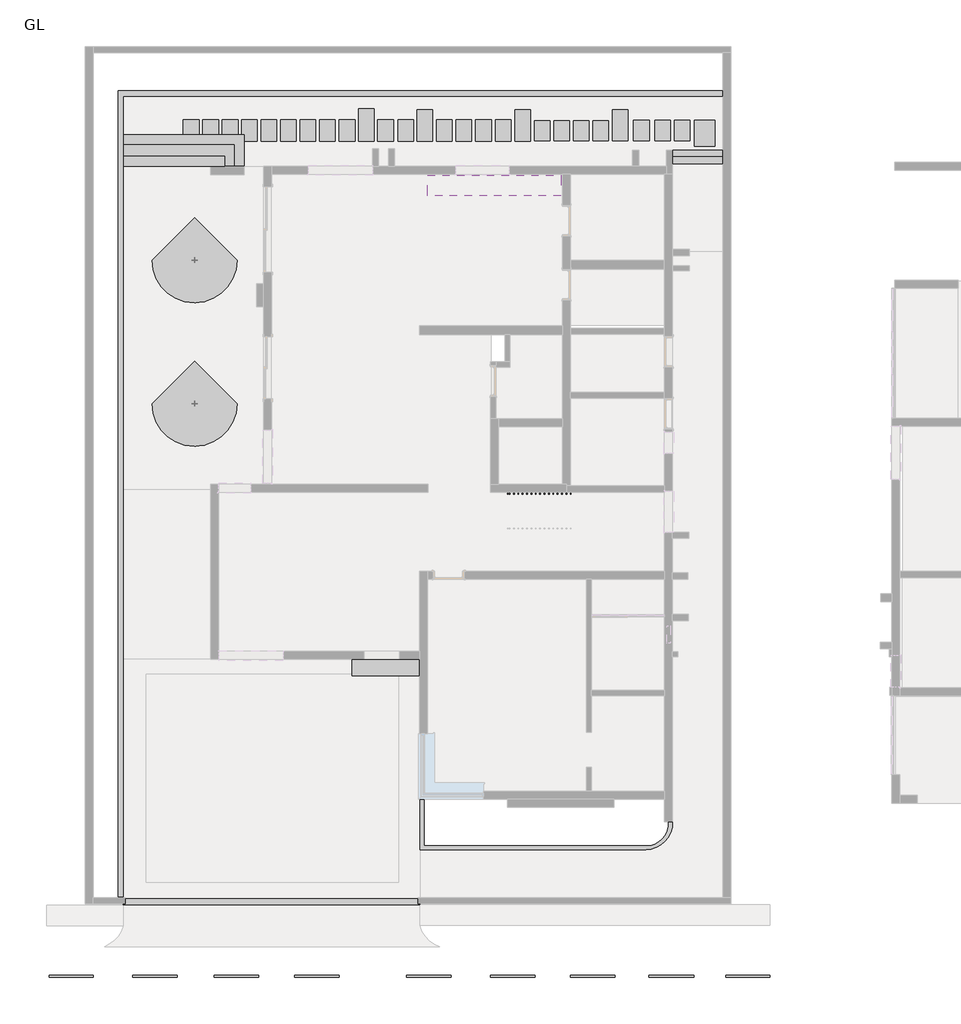
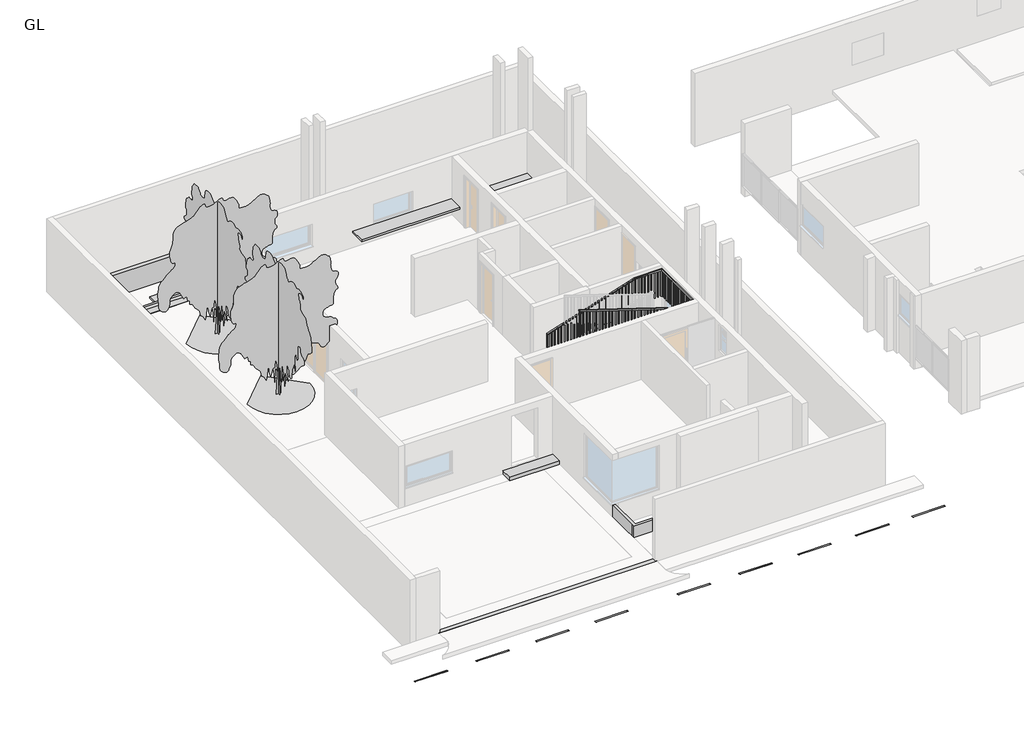
# One storey, part 6 of 6: 5 proxies, 2 geographic elements, 2 stairs, 1 railing.
"""IFC4 building model written with IfcOpenShell, lengths in millimetres."""

from ifc_helpers import new_model, si_unit, frame, origin, place, context, project, spatial, polyline, outline, extrude, faceted_brep, transform, mapped, element, save
from components import generic_models_1_generic_models_1_84634830, generic_models_2_generic_models_2_74674079, generic_models_3_generic_models_3_ad65571d, generic_models_4_generic_models_4_6f48c335, generic_models_5_generic_models_5_efa3826c, planting_rpc_tree_deciduous_golden_chain_5_5_meters_a00e3d8d, stairs_1_stairs_1_bf5218fc, stairs_2_stairs_2_b3d7acac

model = new_model("IFC4")

# Units and contexts
model_context = context("Model", 3, world=origin())
ifc_project = project(units=[si_unit("LENGTHUNIT", "METRE", prefix="MILLI")], contexts=[model_context])

# Site, building, storey
site = spatial("IfcSite", under=ifc_project)
building = spatial("IfcBuilding", under=site)
storey = spatial("IfcBuildingStorey", under=building, Name="GL", Elevation=0.0)

# Proxies
placement = place(None, origin())
generic_models_1_generic_models_1_shape = generic_models_1_generic_models_1_84634830(model_context)
element("IfcBuildingElementProxy", 1, Name="Generic Models 1 : Generic Models 1", ObjectType="Generic Models 1 : Generic Models 1", at=placement, inside=storey, context=model_context, shape_type="MappedRepresentation", body=[
    mapped(generic_models_1_generic_models_1_shape, transform((0.0, 0.0, 0.0), x_axis=(1.0, 0.0, 0.0), y_axis=(0.0, 1.0, 0.0), z_axis=(0.0, 0.0, 1.0))),
])
generic_models_2_generic_models_2_shape = generic_models_2_generic_models_2_74674079(model_context)
element("IfcBuildingElementProxy", 2, Name="Generic Models 2 : Generic Models 2", ObjectType="Generic Models 2 : Generic Models 2", at=placement, inside=storey, context=model_context, shape_type="MappedRepresentation", body=[
    mapped(generic_models_2_generic_models_2_shape, transform((0.0, 0.0, 0.0), x_axis=(1.0, 0.0, 0.0), y_axis=(0.0, 1.0, 0.0), z_axis=(0.0, 0.0, 1.0))),
])
generic_models_3_generic_models_3_shape = generic_models_3_generic_models_3_ad65571d(model_context)
element("IfcBuildingElementProxy", 3, Name="Generic Models 3 : Generic Models 3", ObjectType="Generic Models 3 : Generic Models 3", at=placement, inside=storey, context=model_context, shape_type="MappedRepresentation", body=[
    mapped(generic_models_3_generic_models_3_shape, transform((0.0, 0.0, 0.0), x_axis=(1.0, 0.0, 0.0), y_axis=(0.0, 1.0, 0.0), z_axis=(0.0, 0.0, 1.0))),
])
generic_models_4_generic_models_4_shape = generic_models_4_generic_models_4_6f48c335(model_context)
element("IfcBuildingElementProxy", 4, Name="Generic Models 4 : Generic Models 4", ObjectType="Generic Models 4 : Generic Models 4", at=placement, inside=storey, context=model_context, shape_type="MappedRepresentation", body=[
    mapped(generic_models_4_generic_models_4_shape, transform((0.0, 0.0, 0.0), x_axis=(1.0, 0.0, 0.0), y_axis=(0.0, 1.0, 0.0), z_axis=(0.0, 0.0, 1.0))),
])
generic_models_5_generic_models_5_shape = generic_models_5_generic_models_5_efa3826c(model_context)
element("IfcBuildingElementProxy", 5, Name="Generic Models 5 : Generic Models 5", ObjectType="Generic Models 5 : Generic Models 5", at=placement, inside=storey, context=model_context, shape_type="MappedRepresentation", body=[
    mapped(generic_models_5_generic_models_5_shape, transform((0.0, 0.0, 0.0), x_axis=(1.0, 0.0, 0.0), y_axis=(0.0, 1.0, 0.0), z_axis=(0.0, 0.0, 1.0))),
])

# Geographic elements
planting_rpc_tree_deciduous_golden_chain_5_5_meters_shape = planting_rpc_tree_deciduous_golden_chain_5_5_meters_a00e3d8d(model_context)
element("IfcGeographicElement", 6, ObjectType="Planting_RPC_Tree_Deciduous : Golden_Chain-5.5_Meters", at=placement, inside=storey, context=model_context, shape_type="MappedRepresentation", body=[
    mapped(planting_rpc_tree_deciduous_golden_chain_5_5_meters_shape, transform((-49097.6786333, 20390.8041063, 899.9140625), x_axis=(1.0, 0.0, 0.0), y_axis=(0.0, 1.0, 0.0), z_axis=(0.0, 0.0, 1.0))),
])
element("IfcGeographicElement", 7, ObjectType="Planting_RPC_Tree_Deciduous : Golden_Chain-5.5_Meters", at=placement, inside=storey, context=model_context, shape_type="MappedRepresentation", body=[
    mapped(planting_rpc_tree_deciduous_golden_chain_5_5_meters_shape, transform((-49097.6786333, 24492.9041063, 899.9140625), x_axis=(1.0, 0.0, 0.0), y_axis=(0.0, 1.0, 0.0), z_axis=(0.0, 0.0, 1.0))),
])

# Railing
element("IfcRailing", 8, ObjectType="1100mm", at=placement, inside=storey, context=model_context, shape_type="SolidModel", body=[
    faceted_brep([(-40149.9681829, 17835.7234223, 1799.9767904), (-40149.9681829, 17835.7234223, 1747.4487757), (-40149.9681829, 17785.7234223, 1747.4487757), (-40149.9681829, 17785.7234223, 1799.9767904), (-36733.6681829, 17835.7234223, 2899.9878906), (-36725.8169379, 17835.7234223, 2849.9878906), (-36725.8169379, 17785.7234223, 2849.9878906), (-36733.6681829, 17785.7234223, 2899.9878906), (-35651.74796, 17835.7234223, 2899.9878906), (-35651.74796, 17835.7234223, 2849.9878906), (-35701.74796, 17785.7234223, 2849.9878906), (-35701.74796, 17785.7234223, 2899.9878906), (-35651.74796, 15601.3234223, 2899.9878906), (-35651.74796, 15601.3234223, 2849.9878906), (-35701.74796, 15651.3234223, 2849.9878906), (-35701.74796, 15651.3234223, 2899.9878906), (-36423.0954556, 15601.3234223, 2899.9878906), (-36430.9467006, 15601.3234223, 2849.9878906), (-36430.9467006, 15651.3234223, 2849.9878906), (-36423.0954556, 15651.3234223, 2899.9878906), (-40149.9681829, 15601.3234223, 4100.0), (-40149.9681829, 15651.3234223, 4100.0), (-40149.9681829, 15651.3234223, 4047.4719853), (-40149.9681829, 15601.3234223, 4047.4719853)], [[[0, 1, 2, 3]], [[1, 0, 4, 5]], [[2, 1, 5, 6]], [[3, 2, 6, 7]], [[0, 3, 7, 4]], [[5, 4, 8, 9]], [[6, 5, 9, 10]], [[7, 6, 10, 11]], [[4, 7, 11, 8]], [[9, 8, 12, 13]], [[10, 9, 13, 14]], [[11, 10, 14, 15]], [[8, 11, 15, 12]], [[13, 12, 16, 17]], [[14, 13, 17, 18]], [[15, 14, 18, 19]], [[12, 15, 19, 16]], [[20, 21, 22, 23]], [[17, 16, 20, 23]], [[18, 17, 23, 22]], [[19, 18, 22, 21]], [[16, 19, 21, 20]]]),
    extrude(outline(polyline([(4031.9456028, -40101.74796), (4039.9953284, -40126.74796), (2899.9989909, -40126.74796), (2899.9989909, -40101.74796), (4031.9456028, -40101.74796)])), frame((0.0, 15613.8234223, 0.0), z_axis=(0.0, 1.0, 0.0), x_axis=(0.0, 0.0, 1.0)), (0.0, 0.0, 1.0), 25.0),
    extrude(outline(polyline([(3991.6969749, -39976.74796), (3999.7467005, -40001.74796), (2899.9989909, -40001.74796), (2899.9989909, -39976.74796), (3991.6969749, -39976.74796)])), frame((0.0, 15613.8234223, 0.0), z_axis=(0.0, 1.0, 0.0), x_axis=(0.0, 0.0, 1.0)), (0.0, 0.0, 1.0), 25.0),
    extrude(outline(polyline([(3951.448347, -39851.74796), (3959.4980726, -39876.74796), (2899.9989909, -39876.74796), (2899.9989909, -39851.74796), (3951.448347, -39851.74796)])), frame((0.0, 15613.8234223, 0.0), z_axis=(0.0, 1.0, 0.0), x_axis=(0.0, 0.0, 1.0)), (0.0, 0.0, 1.0), 25.0),
    extrude(outline(polyline([(3911.1997191, -39726.74796), (3919.2494447, -39751.74796), (2799.9979818, -39751.74796), (2799.9979818, -39726.74796), (3911.1997191, -39726.74796)])), frame((0.0, 15613.8234223, 0.0), z_axis=(0.0, 1.0, 0.0), x_axis=(0.0, 0.0, 1.0)), (0.0, 0.0, 1.0), 25.0),
    extrude(outline(polyline([(3870.9510912, -39601.74796), (3879.0008168, -39626.74796), (2799.9979818, -39626.74796), (2799.9979818, -39601.74796), (3870.9510912, -39601.74796)])), frame((0.0, 15613.8234223, 0.0), z_axis=(0.0, 1.0, 0.0), x_axis=(0.0, 0.0, 1.0)), (0.0, 0.0, 1.0), 25.0),
    extrude(outline(polyline([(3830.7024633, -39476.74796), (3838.7521889, -39501.74796), (2699.9969727, -39501.74796), (2699.9969727, -39476.74796), (3830.7024633, -39476.74796)])), frame((0.0, 15613.8234223, 0.0), z_axis=(0.0, 1.0, 0.0), x_axis=(0.0, 0.0, 1.0)), (0.0, 0.0, 1.0), 25.0),
    extrude(outline(polyline([(3790.4538354, -39351.74796), (3798.503561, -39376.74796), (2699.9969727, -39376.74796), (2699.9969727, -39351.74796), (3790.4538354, -39351.74796)])), frame((0.0, 15613.8234223, 0.0), z_axis=(0.0, 1.0, 0.0), x_axis=(0.0, 0.0, 1.0)), (0.0, 0.0, 1.0), 25.0),
    extrude(outline(polyline([(3750.2052075, -39226.74796), (3758.254933, -39251.74796), (2699.9969727, -39251.74796), (2699.9969727, -39226.74796), (3750.2052075, -39226.74796)])), frame((0.0, 15613.8234223, 0.0), z_axis=(0.0, 1.0, 0.0), x_axis=(0.0, 0.0, 1.0)), (0.0, 0.0, 1.0), 25.0),
    extrude(outline(polyline([(3710.0216346, -39101.74796), (3718.0713601, -39126.74796), (2599.9959635, -39126.74796), (2599.9959635, -39101.74796), (3710.0216346, -39101.74796)])), frame((0.0, 15613.8234223, 0.0), z_axis=(0.0, 1.0, 0.0), x_axis=(0.0, 0.0, 1.0)), (0.0, 0.0, 1.0), 25.0),
    extrude(outline(polyline([(3669.7730066, -38976.74796), (3677.8227322, -39001.74796), (2599.9959635, -39001.74796), (2599.9959635, -38976.74796), (3669.7730066, -38976.74796)])), frame((0.0, 15613.8234223, 0.0), z_axis=(0.0, 1.0, 0.0), x_axis=(0.0, 0.0, 1.0)), (0.0, 0.0, 1.0), 25.0),
    extrude(outline(polyline([(3629.5243787, -38851.74796), (3637.5741043, -38876.74796), (2499.9949544, -38876.74796), (2499.9949544, -38851.74796), (3629.5243787, -38851.74796)])), frame((0.0, 15613.8234223, 0.0), z_axis=(0.0, 1.0, 0.0), x_axis=(0.0, 0.0, 1.0)), (0.0, 0.0, 1.0), 25.0),
    extrude(outline(polyline([(3589.2757508, -38726.74796), (3597.3254764, -38751.74796), (2499.9949544, -38751.74796), (2499.9949544, -38726.74796), (3589.2757508, -38726.74796)])), frame((0.0, 15613.8234223, 0.0), z_axis=(0.0, 1.0, 0.0), x_axis=(0.0, 0.0, 1.0)), (0.0, 0.0, 1.0), 25.0),
    extrude(outline(polyline([(3549.0271229, -38601.74796), (3557.0768485, -38626.74796), (2499.9949544, -38626.74796), (2499.9949544, -38601.74796), (3549.0271229, -38601.74796)])), frame((0.0, 15613.8234223, 0.0), z_axis=(0.0, 1.0, 0.0), x_axis=(0.0, 0.0, 1.0)), (0.0, 0.0, 1.0), 25.0),
    extrude(outline(polyline([(3508.778495, -38476.74796), (3516.8282206, -38501.74796), (2399.9939453, -38501.74796), (2399.9939453, -38476.74796), (3508.778495, -38476.74796)])), frame((0.0, 15613.8234223, 0.0), z_axis=(0.0, 1.0, 0.0), x_axis=(0.0, 0.0, 1.0)), (0.0, 0.0, 1.0), 25.0),
    extrude(outline(polyline([(3468.5298671, -38351.74796), (3476.5795927, -38376.74796), (2399.9939453, -38376.74796), (2399.9939453, -38351.74796), (3468.5298671, -38351.74796)])), frame((0.0, 15613.8234223, 0.0), z_axis=(0.0, 1.0, 0.0), x_axis=(0.0, 0.0, 1.0)), (0.0, 0.0, 1.0), 25.0),
    extrude(outline(polyline([(3428.2812392, -38226.74796), (3436.3309648, -38251.74796), (2299.9929362, -38251.74796), (2299.9929362, -38226.74796), (3428.2812392, -38226.74796)])), frame((0.0, 15613.8234223, 0.0), z_axis=(0.0, 1.0, 0.0), x_axis=(0.0, 0.0, 1.0)), (0.0, 0.0, 1.0), 25.0),
    extrude(outline(polyline([(3388.0326113, -38101.74796), (3396.0823368, -38126.74796), (2299.9929362, -38126.74796), (2299.9929362, -38101.74796), (3388.0326113, -38101.74796)])), frame((0.0, 15613.8234223, 0.0), z_axis=(0.0, 1.0, 0.0), x_axis=(0.0, 0.0, 1.0)), (0.0, 0.0, 1.0), 25.0),
    extrude(outline(polyline([(3347.7839834, -37976.74796), (3355.8337089, -38001.74796), (2299.9929362, -38001.74796), (2299.9929362, -37976.74796), (3347.7839834, -37976.74796)])), frame((0.0, 15613.8234223, 0.0), z_axis=(0.0, 1.0, 0.0), x_axis=(0.0, 0.0, 1.0)), (0.0, 0.0, 1.0), 25.0),
    extrude(outline(polyline([(3307.5353554, -37851.74796), (3315.585081, -37876.74796), (2199.9919271, -37876.74796), (2199.9919271, -37851.74796), (3307.5353554, -37851.74796)])), frame((0.0, 15613.8234223, 0.0), z_axis=(0.0, 1.0, 0.0), x_axis=(0.0, 0.0, 1.0)), (0.0, 0.0, 1.0), 25.0),
    extrude(outline(polyline([(3267.2867275, -37726.74796), (3275.3364531, -37751.74796), (2199.9919271, -37751.74796), (2199.9919271, -37726.74796), (3267.2867275, -37726.74796)])), frame((0.0, 15613.8234223, 0.0), z_axis=(0.0, 1.0, 0.0), x_axis=(0.0, 0.0, 1.0)), (0.0, 0.0, 1.0), 25.0),
    extrude(outline(polyline([(3227.0380996, -37601.74796), (3235.0878252, -37626.74796), (2099.990918, -37626.74796), (2099.990918, -37601.74796), (3227.0380996, -37601.74796)])), frame((0.0, 15613.8234223, 0.0), z_axis=(0.0, 1.0, 0.0), x_axis=(0.0, 0.0, 1.0)), (0.0, 0.0, 1.0), 25.0),
    extrude(outline(polyline([(3186.7894717, -37476.74796), (3194.8391973, -37501.74796), (2099.990918, -37501.74796), (2099.990918, -37476.74796), (3186.7894717, -37476.74796)])), frame((0.0, 15613.8234223, 0.0), z_axis=(0.0, 1.0, 0.0), x_axis=(0.0, 0.0, 1.0)), (0.0, 0.0, 1.0), 25.0),
    extrude(outline(polyline([(3146.5408438, -37351.74796), (3154.5905694, -37376.74796), (2099.990918, -37376.74796), (2099.990918, -37351.74796), (3146.5408438, -37351.74796)])), frame((0.0, 15613.8234223, 0.0), z_axis=(0.0, 1.0, 0.0), x_axis=(0.0, 0.0, 1.0)), (0.0, 0.0, 1.0), 25.0),
    extrude(outline(polyline([(3106.2922159, -37226.74796), (3114.3419415, -37251.74796), (1999.9899089, -37251.74796), (1999.9899089, -37226.74796), (3106.2922159, -37226.74796)])), frame((0.0, 15613.8234223, 0.0), z_axis=(0.0, 1.0, 0.0), x_axis=(0.0, 0.0, 1.0)), (0.0, 0.0, 1.0), 25.0),
    extrude(outline(polyline([(3066.043588, -37101.74796), (3074.0933136, -37126.74796), (1999.9899089, -37126.74796), (1999.9899089, -37101.74796), (3066.043588, -37101.74796)])), frame((0.0, 15613.8234223, 0.0), z_axis=(0.0, 1.0, 0.0), x_axis=(0.0, 0.0, 1.0)), (0.0, 0.0, 1.0), 25.0),
    extrude(outline(polyline([(3025.7949601, -36976.74796), (3033.8446856, -37001.74796), (1899.9888997, -37001.74796), (1899.9888997, -36976.74796), (3025.7949601, -36976.74796)])), frame((0.0, 15613.8234223, 0.0), z_axis=(0.0, 1.0, 0.0), x_axis=(0.0, 0.0, 1.0)), (0.0, 0.0, 1.0), 25.0),
    extrude(outline(polyline([(2985.5463322, -36851.74796), (2993.5960577, -36876.74796), (1899.9888997, -36876.74796), (1899.9888997, -36851.74796), (2985.5463322, -36851.74796)])), frame((0.0, 15613.8234223, 0.0), z_axis=(0.0, 1.0, 0.0), x_axis=(0.0, 0.0, 1.0)), (0.0, 0.0, 1.0), 25.0),
    extrude(outline(polyline([(2945.2977042, -36726.74796), (2953.3474298, -36751.74796), (1899.9888997, -36751.74796), (1899.9888997, -36726.74796), (2945.2977042, -36726.74796)])), frame((0.0, 15613.8234223, 0.0), z_axis=(0.0, 1.0, 0.0), x_axis=(0.0, 0.0, 1.0)), (0.0, 0.0, 1.0), 25.0),
    extrude(outline(polyline([(2905.0490763, -36601.74796), (2913.0988019, -36626.74796), (1799.9878906, -36626.74796), (1799.9878906, -36601.74796), (2905.0490763, -36601.74796)])), frame((0.0, 15613.8234223, 0.0), z_axis=(0.0, 1.0, 0.0), x_axis=(0.0, 0.0, 1.0)), (0.0, 0.0, 1.0), 25.0),
    extrude(outline(polyline([(2864.8004484, -36476.74796), (2872.850174, -36501.74796), (1799.9878906, -36501.74796), (1799.9878906, -36476.74796), (2864.8004484, -36476.74796)])), frame((0.0, 15613.8234223, 0.0), z_axis=(0.0, 1.0, 0.0), x_axis=(0.0, 0.0, 1.0)), (0.0, 0.0, 1.0), 25.0),
    extrude(outline(polyline([(-36351.74796, 15613.8234223), (-36376.74796, 15613.8234223), (-36376.74796, 15638.8234223), (-36351.74796, 15638.8234223), (-36351.74796, 15613.8234223)])), frame((0.0, 0.0, 1799.9878906), z_axis=(0.0, 0.0, 1.0), x_axis=(1.0, 0.0, 0.0)), (0.0, 0.0, 1.0), 1050.0),
    extrude(outline(polyline([(-36226.74796, 15613.8234223), (-36251.74796, 15613.8234223), (-36251.74796, 15638.8234223), (-36226.74796, 15638.8234223), (-36226.74796, 15613.8234223)])), frame((0.0, 0.0, 1799.9878906), z_axis=(0.0, 0.0, 1.0), x_axis=(1.0, 0.0, 0.0)), (0.0, 0.0, 1.0), 1050.0),
    extrude(outline(polyline([(-36101.74796, 15613.8234223), (-36126.74796, 15613.8234223), (-36126.74796, 15638.8234223), (-36101.74796, 15638.8234223), (-36101.74796, 15613.8234223)])), frame((0.0, 0.0, 1799.9878906), z_axis=(0.0, 0.0, 1.0), x_axis=(1.0, 0.0, 0.0)), (0.0, 0.0, 1.0), 1050.0),
    extrude(outline(polyline([(-35976.74796, 15613.8234223), (-36001.74796, 15613.8234223), (-36001.74796, 15638.8234223), (-35976.74796, 15638.8234223), (-35976.74796, 15613.8234223)])), frame((0.0, 0.0, 1799.9878906), z_axis=(0.0, 0.0, 1.0), x_axis=(1.0, 0.0, 0.0)), (0.0, 0.0, 1.0), 1050.0),
    extrude(outline(polyline([(-35851.74796, 15613.8234223), (-35876.74796, 15613.8234223), (-35876.74796, 15638.8234223), (-35851.74796, 15638.8234223), (-35851.74796, 15613.8234223)])), frame((0.0, 0.0, 1799.9878906), z_axis=(0.0, 0.0, 1.0), x_axis=(1.0, 0.0, 0.0)), (0.0, 0.0, 1.0), 1050.0),
    extrude(outline(polyline([(-35726.74796, 15613.8234223), (-35751.74796, 15613.8234223), (-35751.74796, 15638.8234223), (-35726.74796, 15638.8234223), (-35726.74796, 15613.8234223)])), frame((0.0, 0.0, 1799.9878906), z_axis=(0.0, 0.0, 1.0), x_axis=(1.0, 0.0, 0.0)), (0.0, 0.0, 1.0), 1050.0),
    extrude(outline(polyline([(-35664.24796, 15760.7234223), (-35664.24796, 15735.7234223), (-35689.24796, 15735.7234223), (-35689.24796, 15760.7234223), (-35664.24796, 15760.7234223)])), frame((0.0, 0.0, 1799.9878906), z_axis=(0.0, 0.0, 1.0), x_axis=(1.0, 0.0, 0.0)), (0.0, 0.0, 1.0), 1050.0),
    extrude(outline(polyline([(-35664.24796, 15885.7234223), (-35664.24796, 15860.7234223), (-35689.24796, 15860.7234223), (-35689.24796, 15885.7234223), (-35664.24796, 15885.7234223)])), frame((0.0, 0.0, 1799.9878906), z_axis=(0.0, 0.0, 1.0), x_axis=(1.0, 0.0, 0.0)), (0.0, 0.0, 1.0), 1050.0),
    extrude(outline(polyline([(-35664.24796, 16010.7234223), (-35664.24796, 15985.7234223), (-35689.24796, 15985.7234223), (-35689.24796, 16010.7234223), (-35664.24796, 16010.7234223)])), frame((0.0, 0.0, 1799.9878906), z_axis=(0.0, 0.0, 1.0), x_axis=(1.0, 0.0, 0.0)), (0.0, 0.0, 1.0), 1050.0),
    extrude(outline(polyline([(-35664.24796, 16135.7234223), (-35664.24796, 16110.7234223), (-35689.24796, 16110.7234223), (-35689.24796, 16135.7234223), (-35664.24796, 16135.7234223)])), frame((0.0, 0.0, 1799.9878906), z_axis=(0.0, 0.0, 1.0), x_axis=(1.0, 0.0, 0.0)), (0.0, 0.0, 1.0), 1050.0),
    extrude(outline(polyline([(-35664.24796, 16260.7234223), (-35664.24796, 16235.7234223), (-35689.24796, 16235.7234223), (-35689.24796, 16260.7234223), (-35664.24796, 16260.7234223)])), frame((0.0, 0.0, 1799.9878906), z_axis=(0.0, 0.0, 1.0), x_axis=(1.0, 0.0, 0.0)), (0.0, 0.0, 1.0), 1050.0),
    extrude(outline(polyline([(-35664.24796, 16385.7234223), (-35664.24796, 16360.7234223), (-35689.24796, 16360.7234223), (-35689.24796, 16385.7234223), (-35664.24796, 16385.7234223)])), frame((0.0, 0.0, 1799.9878906), z_axis=(0.0, 0.0, 1.0), x_axis=(1.0, 0.0, 0.0)), (0.0, 0.0, 1.0), 1050.0),
    extrude(outline(polyline([(-35664.24796, 16510.7234223), (-35664.24796, 16485.7234223), (-35689.24796, 16485.7234223), (-35689.24796, 16510.7234223), (-35664.24796, 16510.7234223)])), frame((0.0, 0.0, 1799.9878906), z_axis=(0.0, 0.0, 1.0), x_axis=(1.0, 0.0, 0.0)), (0.0, 0.0, 1.0), 1050.0),
    extrude(outline(polyline([(-35664.24796, 16635.7234223), (-35664.24796, 16610.7234223), (-35689.24796, 16610.7234223), (-35689.24796, 16635.7234223), (-35664.24796, 16635.7234223)])), frame((0.0, 0.0, 1799.9878906), z_axis=(0.0, 0.0, 1.0), x_axis=(1.0, 0.0, 0.0)), (0.0, 0.0, 1.0), 1050.0),
    extrude(outline(polyline([(-35664.24796, 16760.7234223), (-35664.24796, 16735.7234223), (-35689.24796, 16735.7234223), (-35689.24796, 16760.7234223), (-35664.24796, 16760.7234223)])), frame((0.0, 0.0, 1799.9878906), z_axis=(0.0, 0.0, 1.0), x_axis=(1.0, 0.0, 0.0)), (0.0, 0.0, 1.0), 1050.0),
    extrude(outline(polyline([(-35664.24796, 16885.7234223), (-35664.24796, 16860.7234223), (-35689.24796, 16860.7234223), (-35689.24796, 16885.7234223), (-35664.24796, 16885.7234223)])), frame((0.0, 0.0, 1799.9878906), z_axis=(0.0, 0.0, 1.0), x_axis=(1.0, 0.0, 0.0)), (0.0, 0.0, 1.0), 1050.0),
    extrude(outline(polyline([(-35664.24796, 17010.7234223), (-35664.24796, 16985.7234223), (-35689.24796, 16985.7234223), (-35689.24796, 17010.7234223), (-35664.24796, 17010.7234223)])), frame((0.0, 0.0, 1799.9878906), z_axis=(0.0, 0.0, 1.0), x_axis=(1.0, 0.0, 0.0)), (0.0, 0.0, 1.0), 1050.0),
    extrude(outline(polyline([(-35664.24796, 17135.7234223), (-35664.24796, 17110.7234223), (-35689.24796, 17110.7234223), (-35689.24796, 17135.7234223), (-35664.24796, 17135.7234223)])), frame((0.0, 0.0, 1799.9878906), z_axis=(0.0, 0.0, 1.0), x_axis=(1.0, 0.0, 0.0)), (0.0, 0.0, 1.0), 1050.0),
    extrude(outline(polyline([(-35664.24796, 17260.7234223), (-35664.24796, 17235.7234223), (-35689.24796, 17235.7234223), (-35689.24796, 17260.7234223), (-35664.24796, 17260.7234223)])), frame((0.0, 0.0, 1799.9878906), z_axis=(0.0, 0.0, 1.0), x_axis=(1.0, 0.0, 0.0)), (0.0, 0.0, 1.0), 1050.0),
    extrude(outline(polyline([(-35664.24796, 17385.7234223), (-35664.24796, 17360.7234223), (-35689.24796, 17360.7234223), (-35689.24796, 17385.7234223), (-35664.24796, 17385.7234223)])), frame((0.0, 0.0, 1799.9878906), z_axis=(0.0, 0.0, 1.0), x_axis=(1.0, 0.0, 0.0)), (0.0, 0.0, 1.0), 1050.0),
    extrude(outline(polyline([(-35664.24796, 17510.7234223), (-35664.24796, 17485.7234223), (-35689.24796, 17485.7234223), (-35689.24796, 17510.7234223), (-35664.24796, 17510.7234223)])), frame((0.0, 0.0, 1799.9878906), z_axis=(0.0, 0.0, 1.0), x_axis=(1.0, 0.0, 0.0)), (0.0, 0.0, 1.0), 1050.0),
    extrude(outline(polyline([(-35664.24796, 17635.7234223), (-35664.24796, 17610.7234223), (-35689.24796, 17610.7234223), (-35689.24796, 17635.7234223), (-35664.24796, 17635.7234223)])), frame((0.0, 0.0, 1799.9878906), z_axis=(0.0, 0.0, 1.0), x_axis=(1.0, 0.0, 0.0)), (0.0, 0.0, 1.0), 1050.0),
    extrude(outline(polyline([(-35664.24796, 17760.7234223), (-35664.24796, 17735.7234223), (-35689.24796, 17735.7234223), (-35689.24796, 17760.7234223), (-35664.24796, 17760.7234223)])), frame((0.0, 0.0, 1799.9878906), z_axis=(0.0, 0.0, 1.0), x_axis=(1.0, 0.0, 0.0)), (0.0, 0.0, 1.0), 1050.0),
    extrude(outline(polyline([(-35724.9681829, 17823.2234223), (-35699.9681829, 17823.2234223), (-35699.9681829, 17798.2234223), (-35724.9681829, 17798.2234223), (-35724.9681829, 17823.2234223)])), frame((0.0, 0.0, 1799.9878906), z_axis=(0.0, 0.0, 1.0), x_axis=(1.0, 0.0, 0.0)), (0.0, 0.0, 1.0), 1050.0),
    extrude(outline(polyline([(-35849.9681829, 17823.2234223), (-35824.9681829, 17823.2234223), (-35824.9681829, 17798.2234223), (-35849.9681829, 17798.2234223), (-35849.9681829, 17823.2234223)])), frame((0.0, 0.0, 1799.9878906), z_axis=(0.0, 0.0, 1.0), x_axis=(1.0, 0.0, 0.0)), (0.0, 0.0, 1.0), 1050.0),
    extrude(outline(polyline([(-35974.9681829, 17823.2234223), (-35949.9681829, 17823.2234223), (-35949.9681829, 17798.2234223), (-35974.9681829, 17798.2234223), (-35974.9681829, 17823.2234223)])), frame((0.0, 0.0, 1799.9878906), z_axis=(0.0, 0.0, 1.0), x_axis=(1.0, 0.0, 0.0)), (0.0, 0.0, 1.0), 1050.0),
    extrude(outline(polyline([(-36099.9681829, 17823.2234223), (-36074.9681829, 17823.2234223), (-36074.9681829, 17798.2234223), (-36099.9681829, 17798.2234223), (-36099.9681829, 17823.2234223)])), frame((0.0, 0.0, 1799.9878906), z_axis=(0.0, 0.0, 1.0), x_axis=(1.0, 0.0, 0.0)), (0.0, 0.0, 1.0), 1050.0),
    extrude(outline(polyline([(-36224.9681829, 17823.2234223), (-36199.9681829, 17823.2234223), (-36199.9681829, 17798.2234223), (-36224.9681829, 17798.2234223), (-36224.9681829, 17823.2234223)])), frame((0.0, 0.0, 1799.9878906), z_axis=(0.0, 0.0, 1.0), x_axis=(1.0, 0.0, 0.0)), (0.0, 0.0, 1.0), 1050.0),
    extrude(outline(polyline([(-36349.9681829, 17823.2234223), (-36324.9681829, 17823.2234223), (-36324.9681829, 17798.2234223), (-36349.9681829, 17798.2234223), (-36349.9681829, 17823.2234223)])), frame((0.0, 0.0, 1799.9878906), z_axis=(0.0, 0.0, 1.0), x_axis=(1.0, 0.0, 0.0)), (0.0, 0.0, 1.0), 1050.0),
    extrude(outline(polyline([(-36474.9681829, 17823.2234223), (-36449.9681829, 17823.2234223), (-36449.9681829, 17798.2234223), (-36474.9681829, 17798.2234223), (-36474.9681829, 17823.2234223)])), frame((0.0, 0.0, 1799.9878906), z_axis=(0.0, 0.0, 1.0), x_axis=(1.0, 0.0, 0.0)), (0.0, 0.0, 1.0), 1050.0),
    extrude(outline(polyline([(-36599.9681829, 17823.2234223), (-36574.9681829, 17823.2234223), (-36574.9681829, 17798.2234223), (-36599.9681829, 17798.2234223), (-36599.9681829, 17823.2234223)])), frame((0.0, 0.0, 1799.9878906), z_axis=(0.0, 0.0, 1.0), x_axis=(1.0, 0.0, 0.0)), (0.0, 0.0, 1.0), 1050.0),
    extrude(outline(polyline([(-36724.9681829, 17823.2234223), (-36699.9681829, 17823.2234223), (-36699.9681829, 17798.2234223), (-36724.9681829, 17798.2234223), (-36724.9681829, 17823.2234223)])), frame((0.0, 0.0, 1799.9878906), z_axis=(0.0, 0.0, 1.0), x_axis=(1.0, 0.0, 0.0)), (0.0, 0.0, 1.0), 1050.0),
    extrude(outline(polyline([(1699.9868815, -36849.9681829), (1699.9868815, -36824.9681829), (2818.0622781, -36824.9681829), (2810.0125525, -36849.9681829), (1699.9868815, -36849.9681829)])), frame((0.0, 17798.2234223, 0.0), z_axis=(0.0, 1.0, 0.0), x_axis=(0.0, 0.0, 1.0)), (0.0, 0.0, 1.0), 25.0),
    extrude(outline(polyline([(1699.9868815, -36974.9681829), (1699.9868815, -36949.9681829), (2777.8136502, -36949.9681829), (2769.7639246, -36974.9681829), (1699.9868815, -36974.9681829)])), frame((0.0, 17798.2234223, 0.0), z_axis=(0.0, 1.0, 0.0), x_axis=(0.0, 0.0, 1.0)), (0.0, 0.0, 1.0), 25.0),
    extrude(outline(polyline([(1599.9858724, -37099.9681829), (1599.9858724, -37074.9681829), (2737.5650223, -37074.9681829), (2729.5152967, -37099.9681829), (1599.9858724, -37099.9681829)])), frame((0.0, 17798.2234223, 0.0), z_axis=(0.0, 1.0, 0.0), x_axis=(0.0, 0.0, 1.0)), (0.0, 0.0, 1.0), 25.0),
    extrude(outline(polyline([(1599.9858724, -37224.9681829), (1599.9858724, -37199.9681829), (2697.3163944, -37199.9681829), (2689.2666688, -37224.9681829), (1599.9858724, -37224.9681829)])), frame((0.0, 17798.2234223, 0.0), z_axis=(0.0, 1.0, 0.0), x_axis=(0.0, 0.0, 1.0)), (0.0, 0.0, 1.0), 25.0),
    extrude(outline(polyline([(1599.9858724, -37349.9681829), (1599.9858724, -37324.9681829), (2657.0677665, -37324.9681829), (2649.0180409, -37349.9681829), (1599.9858724, -37349.9681829)])), frame((0.0, 17798.2234223, 0.0), z_axis=(0.0, 1.0, 0.0), x_axis=(0.0, 0.0, 1.0)), (0.0, 0.0, 1.0), 25.0),
    extrude(outline(polyline([(1499.9848633, -37474.9681829), (1499.9848633, -37449.9681829), (2616.8191385, -37449.9681829), (2608.769413, -37474.9681829), (1499.9848633, -37474.9681829)])), frame((0.0, 17798.2234223, 0.0), z_axis=(0.0, 1.0, 0.0), x_axis=(0.0, 0.0, 1.0)), (0.0, 0.0, 1.0), 25.0),
    extrude(outline(polyline([(1499.9848633, -37599.9681829), (1499.9848633, -37574.9681829), (2576.5705106, -37574.9681829), (2568.5207851, -37599.9681829), (1499.9848633, -37599.9681829)])), frame((0.0, 17798.2234223, 0.0), z_axis=(0.0, 1.0, 0.0), x_axis=(0.0, 0.0, 1.0)), (0.0, 0.0, 1.0), 25.0),
    extrude(outline(polyline([(1399.9838542, -37724.9681829), (1399.9838542, -37699.9681829), (2536.3218827, -37699.9681829), (2528.2721571, -37724.9681829), (1399.9838542, -37724.9681829)])), frame((0.0, 17798.2234223, 0.0), z_axis=(0.0, 1.0, 0.0), x_axis=(0.0, 0.0, 1.0)), (0.0, 0.0, 1.0), 25.0),
    extrude(outline(polyline([(1399.9838542, -37849.9681829), (1399.9838542, -37824.9681829), (2496.0732548, -37824.9681829), (2488.0235292, -37849.9681829), (1399.9838542, -37849.9681829)])), frame((0.0, 17798.2234223, 0.0), z_axis=(0.0, 1.0, 0.0), x_axis=(0.0, 0.0, 1.0)), (0.0, 0.0, 1.0), 25.0),
    extrude(outline(polyline([(1399.9838542, -37974.9681829), (1399.9838542, -37949.9681829), (2455.8246269, -37949.9681829), (2447.7749013, -37974.9681829), (1399.9838542, -37974.9681829)])), frame((0.0, 17798.2234223, 0.0), z_axis=(0.0, 1.0, 0.0), x_axis=(0.0, 0.0, 1.0)), (0.0, 0.0, 1.0), 25.0),
    extrude(outline(polyline([(1299.9828451, -38099.9681829), (1299.9828451, -38074.9681829), (2415.575999, -38074.9681829), (2407.5262734, -38099.9681829), (1299.9828451, -38099.9681829)])), frame((0.0, 17798.2234223, 0.0), z_axis=(0.0, 1.0, 0.0), x_axis=(0.0, 0.0, 1.0)), (0.0, 0.0, 1.0), 25.0),
    extrude(outline(polyline([(1299.9828451, -38224.9681829), (1299.9828451, -38199.9681829), (2375.3273711, -38199.9681829), (2367.2776455, -38224.9681829), (1299.9828451, -38224.9681829)])), frame((0.0, 17798.2234223, 0.0), z_axis=(0.0, 1.0, 0.0), x_axis=(0.0, 0.0, 1.0)), (0.0, 0.0, 1.0), 25.0),
    extrude(outline(polyline([(1199.9818359, -38349.9681829), (1199.9818359, -38324.9681829), (2335.0787432, -38324.9681829), (2327.0290176, -38349.9681829), (1199.9818359, -38349.9681829)])), frame((0.0, 17798.2234223, 0.0), z_axis=(0.0, 1.0, 0.0), x_axis=(0.0, 0.0, 1.0)), (0.0, 0.0, 1.0), 25.0),
    extrude(outline(polyline([(1199.9818359, -38474.9681829), (1199.9818359, -38449.9681829), (2294.8301153, -38449.9681829), (2286.7803897, -38474.9681829), (1199.9818359, -38474.9681829)])), frame((0.0, 17798.2234223, 0.0), z_axis=(0.0, 1.0, 0.0), x_axis=(0.0, 0.0, 1.0)), (0.0, 0.0, 1.0), 25.0),
    extrude(outline(polyline([(1199.9818359, -38599.9681829), (1199.9818359, -38574.9681829), (2254.5814873, -38574.9681829), (2246.5317618, -38599.9681829), (1199.9818359, -38599.9681829)])), frame((0.0, 17798.2234223, 0.0), z_axis=(0.0, 1.0, 0.0), x_axis=(0.0, 0.0, 1.0)), (0.0, 0.0, 1.0), 25.0),
    extrude(outline(polyline([(1099.9808268, -38724.9681829), (1099.9808268, -38699.9681829), (2214.3328594, -38699.9681829), (2206.2831339, -38724.9681829), (1099.9808268, -38724.9681829)])), frame((0.0, 17798.2234223, 0.0), z_axis=(0.0, 1.0, 0.0), x_axis=(0.0, 0.0, 1.0)), (0.0, 0.0, 1.0), 25.0),
    extrude(outline(polyline([(1099.9808268, -38849.9681829), (1099.9808268, -38824.9681829), (2174.0842315, -38824.9681829), (2166.0345059, -38849.9681829), (1099.9808268, -38849.9681829)])), frame((0.0, 17798.2234223, 0.0), z_axis=(0.0, 1.0, 0.0), x_axis=(0.0, 0.0, 1.0)), (0.0, 0.0, 1.0), 25.0),
    extrude(outline(polyline([(999.9798177, -38974.9681829), (999.9798177, -38949.9681829), (2133.8356036, -38949.9681829), (2125.785878, -38974.9681829), (999.9798177, -38974.9681829)])), frame((0.0, 17798.2234223, 0.0), z_axis=(0.0, 1.0, 0.0), x_axis=(0.0, 0.0, 1.0)), (0.0, 0.0, 1.0), 25.0),
    extrude(outline(polyline([(999.9798177, -39099.9681829), (999.9798177, -39074.9681829), (2093.5869757, -39074.9681829), (2085.5372501, -39099.9681829), (999.9798177, -39099.9681829)])), frame((0.0, 17798.2234223, 0.0), z_axis=(0.0, 1.0, 0.0), x_axis=(0.0, 0.0, 1.0)), (0.0, 0.0, 1.0), 25.0),
    extrude(outline(polyline([(999.9798177, -39224.9681829), (999.9798177, -39199.9681829), (2053.3383478, -39199.9681829), (2045.2886222, -39224.9681829), (999.9798177, -39224.9681829)])), frame((0.0, 17798.2234223, 0.0), z_axis=(0.0, 1.0, 0.0), x_axis=(0.0, 0.0, 1.0)), (0.0, 0.0, 1.0), 25.0),
    extrude(outline(polyline([(899.9788086, -39349.9681829), (899.9788086, -39324.9681829), (2013.0897199, -39324.9681829), (2005.0399943, -39349.9681829), (899.9788086, -39349.9681829)])), frame((0.0, 17798.2234223, 0.0), z_axis=(0.0, 1.0, 0.0), x_axis=(0.0, 0.0, 1.0)), (0.0, 0.0, 1.0), 25.0),
    extrude(outline(polyline([(899.9788086, -39474.9681829), (899.9788086, -39449.9681829), (1972.841092, -39449.9681829), (1964.7913664, -39474.9681829), (899.9788086, -39474.9681829)])), frame((0.0, 17798.2234223, 0.0), z_axis=(0.0, 1.0, 0.0), x_axis=(0.0, 0.0, 1.0)), (0.0, 0.0, 1.0), 25.0),
    extrude(outline(polyline([(799.9777995, -39599.9681829), (799.9777995, -39574.9681829), (1932.5924641, -39574.9681829), (1924.5427385, -39599.9681829), (799.9777995, -39599.9681829)])), frame((0.0, 17798.2234223, 0.0), z_axis=(0.0, 1.0, 0.0), x_axis=(0.0, 0.0, 1.0)), (0.0, 0.0, 1.0), 25.0),
    extrude(outline(polyline([(799.9777995, -39724.9681829), (799.9777995, -39699.9681829), (1892.3438361, -39699.9681829), (1884.2941106, -39724.9681829), (799.9777995, -39724.9681829)])), frame((0.0, 17798.2234223, 0.0), z_axis=(0.0, 1.0, 0.0), x_axis=(0.0, 0.0, 1.0)), (0.0, 0.0, 1.0), 25.0),
    extrude(outline(polyline([(799.9777995, -39849.9681829), (799.9777995, -39824.9681829), (1852.0952082, -39824.9681829), (1844.0454827, -39849.9681829), (799.9777995, -39849.9681829)])), frame((0.0, 17798.2234223, 0.0), z_axis=(0.0, 1.0, 0.0), x_axis=(0.0, 0.0, 1.0)), (0.0, 0.0, 1.0), 25.0),
    extrude(outline(polyline([(699.9767904, -39974.9681829), (699.9767904, -39949.9681829), (1811.8465803, -39949.9681829), (1803.7968547, -39974.9681829), (699.9767904, -39974.9681829)])), frame((0.0, 17798.2234223, 0.0), z_axis=(0.0, 1.0, 0.0), x_axis=(0.0, 0.0, 1.0)), (0.0, 0.0, 1.0), 25.0),
    extrude(outline(polyline([(699.9767904, -40099.9681829), (699.9767904, -40074.9681829), (1771.5979524, -40074.9681829), (1763.5482268, -40099.9681829), (699.9767904, -40099.9681829)])), frame((0.0, 17798.2234223, 0.0), z_axis=(0.0, 1.0, 0.0), x_axis=(0.0, 0.0, 1.0)), (0.0, 0.0, 1.0), 25.0),
    extrude(outline(polyline([(-35664.24796, 15638.8234223), (-35664.24796, 15613.8234223), (-35689.24796, 15613.8234223), (-35689.24796, 15638.8234223), (-35664.24796, 15638.8234223)])), frame((0.0, 0.0, 1799.9878906), z_axis=(0.0, 0.0, 1.0), x_axis=(1.0, 0.0, 0.0)), (0.0, 0.0, 1.0), 1050.0),
    extrude(outline(polyline([(-35689.24796, 17823.2234223), (-35664.24796, 17823.2234223), (-35664.24796, 17798.2234223), (-35689.24796, 17798.2234223), (-35689.24796, 17823.2234223)])), frame((0.0, 0.0, 1799.9878906), z_axis=(0.0, 0.0, 1.0), x_axis=(1.0, 0.0, 0.0)), (0.0, 0.0, 1.0), 1050.0),
    extrude(outline(polyline([(4039.4222597, -40124.9681829), (4047.4719853, -40149.9681829), (2899.9989909, -40149.9681829), (2899.9989909, -40124.9681829), (4039.4222597, -40124.9681829)])), frame((0.0, 15613.8234223, 0.0), z_axis=(0.0, 1.0, 0.0), x_axis=(0.0, 0.0, 1.0)), (0.0, 0.0, 1.0), 25.0),
    extrude(outline(polyline([(699.9767904, -40149.9681829), (699.9767904, -40124.9681829), (1755.4985013, -40124.9681829), (1747.4487757, -40149.9681829), (699.9767904, -40149.9681829)])), frame((0.0, 17798.2234223, 0.0), z_axis=(0.0, 1.0, 0.0), x_axis=(0.0, 0.0, 1.0)), (0.0, 0.0, 1.0), 25.0),
])

# Stairs
stairs_1_stairs_1_shape = stairs_1_stairs_1_bf5218fc(model_context)
element("IfcStair", 9, ObjectType="Stairs 1 : Stairs 1", at=placement, inside=storey, context=model_context, shape_type="MappedRepresentation", body=[
    mapped(stairs_1_stairs_1_shape, transform((0.0, 0.0, 0.0), x_axis=(1.0, 0.0, 0.0), y_axis=(0.0, 1.0, 0.0), z_axis=(0.0, 0.0, 1.0))),
])
stairs_2_stairs_2_shape = stairs_2_stairs_2_b3d7acac(model_context)
element("IfcStair", 10, ObjectType="Stairs 2 : Stairs 2", at=placement, inside=storey, context=model_context, shape_type="MappedRepresentation", body=[
    mapped(stairs_2_stairs_2_shape, transform((0.0, 0.0, 0.0), x_axis=(1.0, 0.0, 0.0), y_axis=(0.0, 1.0, 0.0), z_axis=(0.0, 0.0, 1.0))),
])

save(model, "model.ifc")

# Revit data of these elements
# Type "Planting_RPC_Tree_Deciduous : Golden_Chain-5.5_Meters"
#   built-in parameter 1005198 = "{2, 15},{39, RPC-16-FXGQ-QK7X-PJ74-6000-ST1L-LVER-AU},{1, 0},{1, 0},{2, 35},{1, 8},{5, Color},{1, 0},{1, 0},{3, 0.8},{3, 0.8},{3, 0.8},{1, 8},{7, BBoxMin},{1, 0},{1, 0},{1, 0},{1, 0},{1, 0},{1, 8},{7, BBoxMax},{1, 0},{1, 0},{1, 0},{1, 0},{1, 0},{2, 11},{9, RPCTypeId},{1, 0},{1, 0},{39, RPC-16-FXGQ-QK7X-PJ74-6000-ST1L-LVER-AU},{1, 6},{14, RPCPlantHeight},{1, 0},{1, 0},{7, 18.0446},{2, 11},{7, keyword},{1, 0},{1, 0},{140, :Geometry:RPC:Golden-chain :Laburnum:Laburnums are very small trees native to southern Europe.  The common cultivar in Canada is 'Watereri'.},{2, 11},{8, category},{1, 0},{1, 0},{16, :Trees [General]},{2, 11},{12, LocalizedUID},{1, 0},{1, 0},{13, Golden-chain },{2, 14},{6, Height},{1, 0},{1, 0},{7, 18.0446},{1, 2},{16, Cast Reflections},{1, 0},{1, 0},{1, 0},{1, 2},{12, Cast Shadows},{1, 0},{1, 0},{1, 1},{1, 2},{9, Lock View},{1, 0},{1, 0},{1, 0},{1, 4},{5, ViewC},{1, 0},{1, 0},{1, 0},{2, 11},{20, AdvancedUIDefinition},{1, 0},{1, 0},{0, },{2, 11},{10, AssetLibID},{1, 0},{1, 0},{36, 4D3F6E72-3F99-4203-98E9-AF80B3C7A7A4},{2, 11},{10, BaseSchema},{1, 0},{1, 0},{9, RPCSchema},{2, 11},{12, ExchangeGUID},{1, 0},{1, 0},{0, },{1, 2},{6, Hidden},{1, 0},{1, 0},{1, 0},{1, 4},{11, RPCCategory},{1, 0},{1, 0},{1, 0},{2, 11},{8, RPCImage},{1, 0},{1, 0},{0, },{1, 4},{13, SchemaVersion},{1, 0},{1, 0},{1, 4},{2, 11},{12, UIDefinition},{1, 0},{1, 0},{0, },{2, 11},{6, UIName},{1, 0},{1, 0},{39, RPC-16-FXGQ-QK7X-PJ74-6000-ST1L-LVER-AU},{2, 11},{11, VersionGUID},{1, 0},{1, 0},{9, RPCSchema},{2, 11},{9, assettype},{1, 0},{1, 0},{11, RPCGeometry},{2, 11},{11, description},{1, 0},{1, 0},{0, },{2, 11},{9, localname},{1, 0},{1, 0},{3, RPC},{2, 11},{9, localtype},{1, 0},{1, 0},{3, RPC},{1, 4},{8, revision},{1, 0},{1, 0},{1, 1},{2, 11},{9, thumbnail},{1, 0},{1, 0},{0, },{1, 4},{7, version},{1, 0},{1, 0},{1, 1},{1, 2},{20, RPC_Cast Reflections},{1, 0},{1, 0},{1, 1},{1, 2},{16, RPC_Cast Shadows},{1, 0},{1, 0},{1, 1},{1, 2},{13, RPC_Lock View},{1, 0},{1, 0},{1, 0},{1, 4},{9, RPC_ViewC},{1, 0},{1, 0},{1, 0},{21, assetlibrary_base.fbx},{1, 5},"
#   built-in parameter 1005195 = "RPC-16-FXGQ-QK7X-PJ74-6000-ST1L-LVER-AU"
#   Type Comments = "Golden Chain"
#   Height = 18' - 0.53543"
#   Default Elevation = 0
# Type "1100mm"
#   built-in parameter 1008612 = 0.019685 (stored number, unit not read)
#   built-in parameter 1008611 = 0.019685 (stored number, unit not read)
#   built-in parameter 1008609 = 0.902231 (stored number, unit not read)
#   built-in parameter 1008604 = 0.19685 (stored number, unit not read)
#   built-in parameter 1008603 = 0.164042 (stored number, unit not read)
#   Railing Height = 3' - 7.30709"
#   built-in parameter 1008630 = 2
#   built-in parameter 1008610 = 2
#   built-in parameter 1008608 = 1
#   built-in parameter 1008618 = Baluster_Square : 25mm
# Element 1 (IfcBuildingElementProxy, "Generic Models 1 : Generic Models 1")
#   Phase Created = New Construction
# Element 2 (IfcBuildingElementProxy, "Generic Models 2 : Generic Models 2")
#   Phase Created = New Construction
# Element 3 (IfcBuildingElementProxy, "Generic Models 3 : Generic Models 3")
#   Phase Created = New Construction
# Element 4 (IfcBuildingElementProxy, "Generic Models 4 : Generic Models 4")
#   Phase Created = New Construction
# Element 5 (IfcBuildingElementProxy, "Generic Models 5 : Generic Models 5")
#   Phase Created = New Construction
# Elements 6, 7 (IfcGeographicElement, "Planting_RPC_Tree_Deciduous : Golden_Chain-5.5_Meters")
#   Phase Created = New Construction
# Element 8 (IfcRailing, "1100mm")
#   Phase Created = New Construction
# Element 9 (IfcStair, "Stairs 1 : Stairs 1")
#   Phase Created = New Construction
# Element 10 (IfcStair, "Stairs 2 : Stairs 2")
#   Phase Created = New Construction
